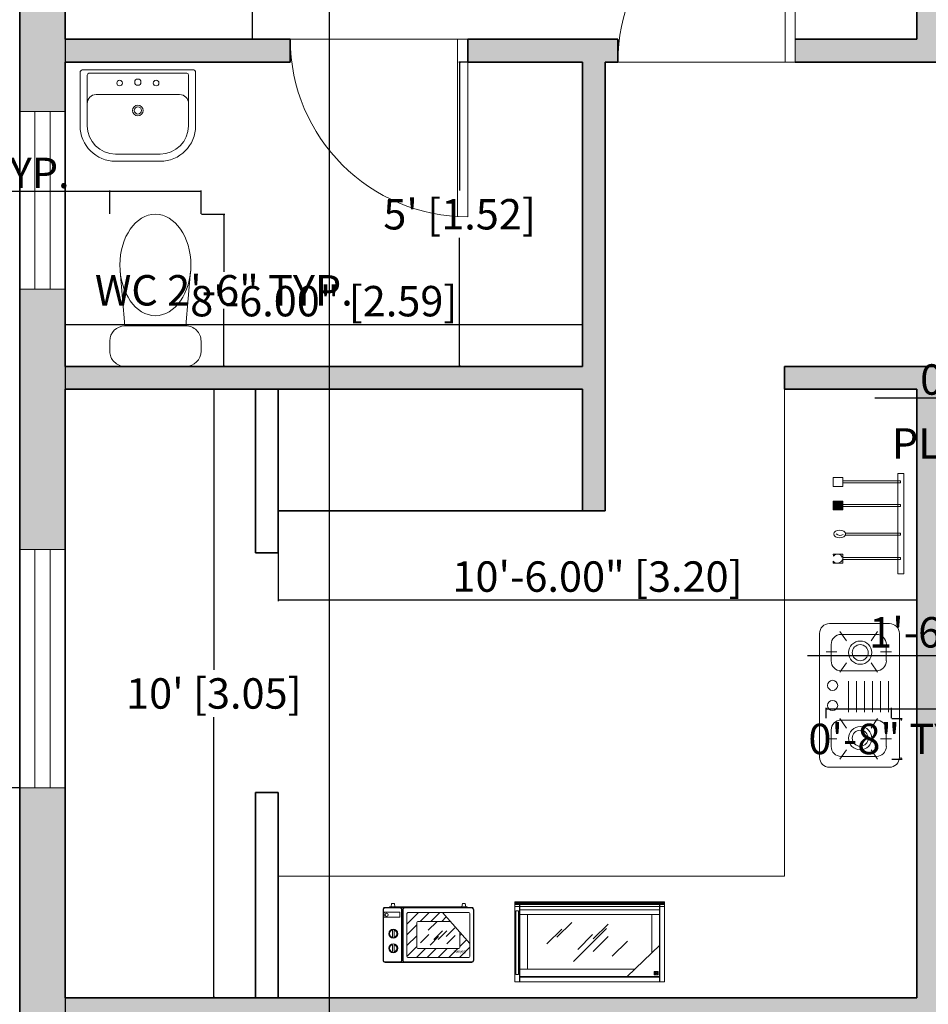
# Model space of a CAD drawing. Units: inches. Extents: x 2322 to 2932, y 142 to 762.
# Tile 4 of 7: x 2430 to 2609, y 376 to 570. Entities that reach past the tile are written whole.
import ezdxf

# ---------------------------------------------------------------- set-up
doc = ezdxf.new("R2010")
doc.units = ezdxf.units.IN
doc.header["$MEASUREMENT"] = 0
for name, color, linetype, lineweight in [('A-ANNO-DIMS', 2, 'Continuous', 18), ('A-ANNO-TEXT', 7, 'Continuous', 15), ('A-DOOR', 3, 'Continuous', 18), ('A-EQPM', 8, 'Continuous', 15), ('A-EQPM-PATT', 8, 'Continuous', 13), ('A-FLOR-CASE', 32, 'Continuous', 18), ('A-FLOR-FIXT', 9, 'Continuous', 18), ('A-GLAZ', 4, 'Continuous', 18), ('A-WALL', 7, 'Continuous', 35)]:
    doc.layers.add(name, color=color, linetype=linetype, lineweight=lineweight)
doc.layers.add('A-WALL-PATT', color=40, linetype='Continuous', lineweight=13, true_color=0xf8d731)
doc.styles.get("Standard").update_dxf_attribs({"font": 'italic8.shx'})
doc.dimstyles.get("Standard").update_dxf_attribs({"dimtxt": 6, "dimasz": 0.15, "dimexe": 0.18, "dimexo": 0.0625, "dimgap": 0.09, "dimtad": 1, "dimtih": 1, "dimtoh": 1, "dimzin": 0, "dimdsep": 46, "dimlunit": 3, "dimtxsty": 'Standard', "dimblk": 'CLOSEDBLANK', "dimcen": 0.09, "dimclrd": 3, "dimclre": 1, "dimclrt": 6, "dimadec": 0, "dimazin": 0, "dimtfac": 1, "dimtofl": 0, "dimtmove": 0, "dimatfit": 3, "dimldrblk": 'DOT', "dimfxl": 1, "dimtolj": 1, "dimtzin": 0, "dimarcsym": 0})

# ---------------------------------------------------------------- blocks, each defined once
blk = doc.blocks.new('_ClosedBlank')
at = {"color": 0, "linetype": 'ByBlock', "lineweight": -2}
for p, q in [((-1, 0.2), (0, 0)), ((-1, 0.2), (-1, -0.2)), ((0, 0), (-1, -0.2))]:
    blk.add_line(p, q, dxfattribs=at)
blk = doc.blocks.new('*D8')
at = {"layer": 'A-ANNO-DIMS', "color": 0, "lineweight": -2, "transparency": 16777216}
for p, q in [((2430, 718.82), (2352.33, 718.82)), ((2352.51, 718.67), (2352.51, 501.45)), ((2352.51, 274.91), (2352.51, 492.13)), ((2430, 274.76), (2352.33, 274.76))]:
    blk.add_line(p, q, dxfattribs=at)
at = {"layer": 'Defpoints', "color": 0, "transparency": 16777216}
for p in [(2430.06, 718.82), (2352.51, 274.76), (2430.06, 274.76)]:
    blk.add_point(p, dxfattribs=at)
at = {"layer": 'A-ANNO-DIMS', "color": 0, "lineweight": -2, "transparency": 16777216, "xscale": 0.15, "yscale": 0.15, "zscale": 0.15}
for p, rotation in [((2352.51, 718.82), 90), ((2352.51, 274.76), 270)]:
    blk.add_blockref('_ClosedBlank', p, dxfattribs=dict(at, rotation=rotation))
at = {"layer": 'A-ANNO-DIMS', "color": 0, "transparency": 16777216, "insert": (2352.51, 496.79), "char_height": 6, "attachment_point": 5}
blk.add_mtext('\\A1;37\'-0.06" [11.28]', dxfattribs=at)
blk = doc.blocks.new('_Dot')
at = {"color": 0, "linetype": 'ByBlock', "lineweight": -2}
blk.add_line((-0.5, 0), (-1, 0), dxfattribs=at)
at = {"color": 0, "linetype": 'ByBlock', "const_width": 0.5}
blk.add_lwpolyline([(-0.25, 0, 1), (0.25, 0, 1)], format="xyb", close=True, dxfattribs=at)
blk = doc.blocks.new('*D9')
at = {"layer": 'A-ANNO-DIMS', "color": 0, "lineweight": -2, "transparency": 16777216}
for p, q in [((2460.73, 709.82), (2476.2, 709.82)), ((2476.02, 709.67), (2476.02, 642.48)), ((2476.02, 565.97), (2476.02, 633.16)), ((2460.73, 565.82), (2476.2, 565.82))]:
    blk.add_line(p, q, dxfattribs=at)
at = {"layer": 'Defpoints', "color": 0, "transparency": 16777216}
for p in [(2460.67, 709.82), (2460.67, 565.82), (2476.02, 565.82)]:
    blk.add_point(p, dxfattribs=at)
at = {"layer": 'A-ANNO-DIMS', "color": 0, "lineweight": -2, "transparency": 16777216, "xscale": 0.15, "yscale": 0.15, "zscale": 0.15}
for p, rotation in [((2476.02, 709.82), 90), ((2476.02, 565.82), 270)]:
    blk.add_blockref('_ClosedBlank', p, dxfattribs=dict(at, rotation=rotation))
at = {"layer": 'A-ANNO-DIMS', "color": 0, "transparency": 16777216, "insert": (2476.02, 637.82), "char_height": 6, "attachment_point": 5}
blk.add_mtext("\\A1;12' [3.66]", dxfattribs=at)
blk = doc.blocks.new('*D14')
at = {"layer": 'A-ANNO-DIMS', "color": 0, "lineweight": -2, "transparency": 16777216}
for p, q in [((2439.06, 531.26), (2439.06, 509.34)), ((2541.06, 531.26), (2541.06, 509.34)), ((2540.91, 509.52), (2439.21, 509.52))]:
    blk.add_line(p, q, dxfattribs=at)
at = {"layer": 'Defpoints', "color": 0, "transparency": 16777216}
for p in [(2439.06, 531.32), (2541.06, 531.32), (2439.06, 509.52)]:
    blk.add_point(p, dxfattribs=at)
at = {"layer": 'A-ANNO-DIMS', "color": 0, "lineweight": -2, "transparency": 16777216, "xscale": 0.15, "yscale": 0.15, "zscale": 0.15, "rotation": 180}
blk.add_blockref('_ClosedBlank', (2439.06, 509.52), dxfattribs=at)
at = {"layer": 'A-ANNO-DIMS', "color": 0, "lineweight": -2, "transparency": 16777216, "xscale": 0.15, "yscale": 0.15, "zscale": 0.15}
blk.add_blockref('_ClosedBlank', (2541.06, 509.52), dxfattribs=at)
at = {"layer": 'A-ANNO-DIMS', "color": 0, "transparency": 16777216, "insert": (2490.06, 514.18), "char_height": 6, "attachment_point": 5}
blk.add_mtext('\\A1;8\'-6.00" [2.59]', dxfattribs=at)
blk = doc.blocks.new('*D15')
at = {"layer": 'A-ANNO-DIMS', "color": 0, "lineweight": -2, "transparency": 16777216}
for p, q in [((2525.45, 561.32), (2516.67, 561.32)), ((2516.85, 561.17), (2516.85, 535.98)), ((2516.85, 501.47), (2516.85, 526.66)), ((2525.45, 501.32), (2516.67, 501.32))]:
    blk.add_line(p, q, dxfattribs=at)
at = {"layer": 'Defpoints', "color": 0, "transparency": 16777216}
for p in [(2525.51, 561.32), (2516.85, 501.32), (2525.51, 501.32)]:
    blk.add_point(p, dxfattribs=at)
at = {"layer": 'A-ANNO-DIMS', "color": 0, "lineweight": -2, "transparency": 16777216, "xscale": 0.15, "yscale": 0.15, "zscale": 0.15}
for p, rotation in [((2516.85, 561.32), 90), ((2516.85, 501.32), 270)]:
    blk.add_blockref('_ClosedBlank', p, dxfattribs=dict(at, rotation=rotation))
at = {"layer": 'A-ANNO-DIMS', "color": 0, "transparency": 16777216, "insert": (2516.85, 531.32), "char_height": 6, "attachment_point": 5}
blk.add_mtext("\\A1;5' [1.52]", dxfattribs=at)
blk = doc.blocks.new('*D16')
at = {"layer": 'A-ANNO-DIMS', "color": 0, "lineweight": -2, "transparency": 16777216}
for p, q in [((2481.06, 469.54), (2481.06, 455.03)), ((2607.06, 469.54), (2607.06, 455.03)), ((2606.91, 455.21), (2481.21, 455.21))]:
    blk.add_line(p, q, dxfattribs=at)
at = {"layer": 'Defpoints', "color": 0, "transparency": 16777216}
for p in [(2481.06, 469.6), (2607.06, 469.6), (2481.06, 455.21)]:
    blk.add_point(p, dxfattribs=at)
at = {"layer": 'A-ANNO-DIMS', "color": 0, "lineweight": -2, "transparency": 16777216, "xscale": 0.15, "yscale": 0.15, "zscale": 0.15, "rotation": 180}
blk.add_blockref('_ClosedBlank', (2481.06, 455.21), dxfattribs=at)
at = {"layer": 'A-ANNO-DIMS', "color": 0, "lineweight": -2, "transparency": 16777216, "xscale": 0.15, "yscale": 0.15, "zscale": 0.15}
blk.add_blockref('_ClosedBlank', (2607.06, 455.21), dxfattribs=at)
at = {"layer": 'A-ANNO-DIMS', "color": 0, "transparency": 16777216, "insert": (2544.06, 459.87), "char_height": 6, "attachment_point": 5}
blk.add_mtext('\\A1;10\'-6.00" [3.20]', dxfattribs=at)
blk = doc.blocks.new('*D17')
at = {"layer": 'A-ANNO-DIMS', "color": 0, "lineweight": -2, "transparency": 16777216}
for p, q in [((2460.37, 496.82), (2468.55, 496.82)), ((2468.37, 496.67), (2468.37, 441.48)), ((2468.37, 376.97), (2468.37, 432.16)), ((2460.37, 376.82), (2468.55, 376.82))]:
    blk.add_line(p, q, dxfattribs=at)
at = {"layer": 'Defpoints', "color": 0, "transparency": 16777216}
for p in [(2460.31, 496.82), (2460.31, 376.82), (2468.37, 376.82)]:
    blk.add_point(p, dxfattribs=at)
at = {"layer": 'A-ANNO-DIMS', "color": 0, "lineweight": -2, "transparency": 16777216, "xscale": 0.15, "yscale": 0.15, "zscale": 0.15}
for p, rotation in [((2468.37, 496.82), 90), ((2468.37, 376.82), 270)]:
    blk.add_blockref('_ClosedBlank', p, dxfattribs=dict(at, rotation=rotation))
at = {"layer": 'A-ANNO-DIMS', "color": 0, "transparency": 16777216, "insert": (2468.37, 436.82), "char_height": 6, "attachment_point": 5}
blk.add_mtext("\\A1;10' [3.05]", dxfattribs=at)
blk = doc.blocks.new('DOOR-SWING-35')
for p, q in [((0, 35), (0, 0)), ((2, 35), (2, 0)), ((0, 0), (35, 0))]:
    blk.add_line(p, q)
blk.add_arc((0, 0), 35, 0, 90)
blk = doc.blocks.new('WINDOW-47X9')
for p, q in [((47, 9), (0, 9)), ((0, 9), (0, 0)), ((47, 0), (47, 9)), ((0, 6), (47, 6)), ((0, 3), (47, 3)), ((0, 0), (47, 0))]:
    blk.add_line(p, q)
blk = doc.blocks.new('WC-TANK')
for p, q in [((3, 18), (5, 18)), ((8, 15), (18.75, 15.95)), ((0, 3), (0, 15)), ((8, 15), (8, 3)), ((8, 3), (18.75, 2.05)), ((5, 0), (3, 0))]:
    blk.add_line(p, q)
for centre, start, end in [((3, 15), 90, 180), ((5, 15), 0, 90), ((3, 3), 180, 270), ((5, 3), 270, 0)]:
    blk.add_arc(centre, 3, start, end)
blk.add_ellipse((20, 9), major_axis=(10, 0), ratio=0.7)
blk = doc.blocks.new('COOKTOP-BURNER')
for p, q in [((2.72, 8.03), (4.01, 6.17)), ((10.17, 8.03), (8.88, 6.17)), ((9.92, 7.46), (2.97, 7.46)), ((0, 4.01), (2.15, 4.01)), ((1, 5.49), (1, 2.25)), ((12.89, 4.01), (10.74, 4.01)), ((11.88, 2.25), (11.88, 5.49)), ((2.72, 0), (4.01, 1.86)), ((2.97, 0.29), (9.92, 0.29)), ((10.17, 0), (8.88, 1.86))]:
    blk.add_line(p, q)
for radius in [2.29, 1.58]:
    blk.add_circle((6.73, 3.87), radius)
for centre, start, end in [((2.97, 5.49), 90, 180), ((9.92, 5.49), 0, 90), ((2.97, 2.25), 180, 270), ((9.92, 2.25), 270, 0)]:
    blk.add_arc(centre, 1.97, start, end)
blk = doc.blocks.new('*D31')
at = {"layer": 'A-ANNO-DIMS', "color": 1, "lineweight": -2, "transparency": 16777216}
for p, q in [((2660.69, 447.24), (2660.69, 444.03)), ((2679.17, 447.24), (2679.17, 444.03))]:
    blk.add_line(p, q, dxfattribs=at)
at = {"layer": 'A-ANNO-DIMS', "color": 3, "lineweight": -2, "transparency": 16777216}
for p, q in [((2660.69, 444.21), (2585.5, 444.21)), ((2679.02, 444.21), (2660.84, 444.21))]:
    blk.add_line(p, q, dxfattribs=at)
at = {"layer": 'Defpoints', "color": 0, "transparency": 16777216}
for p in [(2660.69, 447.3), (2679.17, 447.3), (2660.69, 444.21)]:
    blk.add_point(p, dxfattribs=at)
at = {"layer": 'A-ANNO-DIMS', "color": 3, "lineweight": -2, "transparency": 16777216, "xscale": 0.15, "yscale": 0.15, "zscale": 0.15, "rotation": 180}
blk.add_blockref('_ClosedBlank', (2660.69, 444.21), dxfattribs=at)
at = {"layer": 'A-ANNO-DIMS', "color": 3, "lineweight": -2, "transparency": 16777216, "xscale": 0.15, "yscale": 0.15, "zscale": 0.15}
blk.add_blockref('_ClosedBlank', (2679.17, 444.21), dxfattribs=at)
at = {"layer": 'A-ANNO-DIMS', "color": 6, "transparency": 16777216, "insert": (2623.02, 448.87), "char_height": 6, "attachment_point": 5}
blk.add_mtext('\\A1;1\'-6 1/2" TYP.', dxfattribs=at)
blk = doc.blocks.new('*D32')
at = {"layer": 'A-ANNO-DIMS', "color": 1, "lineweight": -2, "transparency": 16777216}
for p, q in [((2653.34, 493), (2651.16, 493)), ((2653.34, 479.24), (2651.16, 479.24))]:
    blk.add_line(p, q, dxfattribs=at)
at = {"layer": 'A-ANNO-DIMS', "color": 3, "lineweight": -2, "transparency": 16777216}
for p, q in [((2651.34, 492.85), (2651.34, 489.78)), ((2651.34, 479.39), (2651.34, 482.46))]:
    blk.add_line(p, q, dxfattribs=at)
at = {"layer": 'Defpoints', "color": 0, "transparency": 16777216}
for p in [(2653.4, 493), (2651.34, 479.24), (2653.4, 479.24)]:
    blk.add_point(p, dxfattribs=at)
at = {"layer": 'A-ANNO-DIMS', "color": 3, "lineweight": -2, "transparency": 16777216, "xscale": 0.15, "yscale": 0.15, "zscale": 0.15}
for p, rotation in [((2651.34, 493), 90), ((2651.34, 479.24), 270)]:
    blk.add_blockref('_ClosedBlank', p, dxfattribs=dict(at, rotation=rotation))
at = {"layer": 'A-ANNO-DIMS', "color": 6, "transparency": 16777216, "insert": (2651.34, 486.12), "char_height": 6, "attachment_point": 5}
blk.add_mtext('\\A1;PLACE SETTING 1\'-2" TYP.', dxfattribs=at)
blk = doc.blocks.new('*D33')
at = {"layer": 'A-ANNO-DIMS', "color": 1, "lineweight": -2, "transparency": 16777216}
for p, q in [((2653.4, 493.07), (2653.4, 495.25)), ((2662.31, 493.07), (2662.31, 495.25))]:
    blk.add_line(p, q, dxfattribs=at)
at = {"layer": 'A-ANNO-DIMS', "color": 3, "lineweight": -2, "transparency": 16777216}
for p, q in [((2653.4, 495.07), (2598.79, 495.07)), ((2662.16, 495.07), (2653.55, 495.07))]:
    blk.add_line(p, q, dxfattribs=at)
at = {"layer": 'Defpoints', "color": 0, "transparency": 16777216}
for p in [(2653.4, 495.07), (2653.4, 493), (2662.31, 493)]:
    blk.add_point(p, dxfattribs=at)
at = {"layer": 'A-ANNO-DIMS', "color": 3, "lineweight": -2, "transparency": 16777216, "xscale": 0.15, "yscale": 0.15, "zscale": 0.15, "rotation": 180}
blk.add_blockref('_ClosedBlank', (2653.4, 495.07), dxfattribs=at)
at = {"layer": 'A-ANNO-DIMS', "color": 3, "lineweight": -2, "transparency": 16777216, "xscale": 0.15, "yscale": 0.15, "zscale": 0.15}
blk.add_blockref('_ClosedBlank', (2662.31, 495.07), dxfattribs=at)
at = {"layer": 'A-ANNO-DIMS', "color": 6, "transparency": 16777216, "insert": (2626.02, 498.73), "char_height": 6, "attachment_point": 5}
blk.add_mtext('\\A1;0\'-9" TYP.', dxfattribs=at)
blk = doc.blocks.new('*D36')
at = {"layer": 'A-ANNO-DIMS', "color": 1, "lineweight": -2, "transparency": 16777216}
for p, q in [((2465.9, 531.32), (2470.52, 531.32)), ((2465.9, 501.32), (2470.52, 501.32))]:
    blk.add_line(p, q, dxfattribs=at)
at = {"layer": 'A-ANNO-DIMS', "color": 3, "lineweight": -2, "transparency": 16777216}
for p, q in [((2470.34, 531.17), (2470.34, 519.98)), ((2470.34, 501.47), (2470.34, 512.66))]:
    blk.add_line(p, q, dxfattribs=at)
at = {"layer": 'Defpoints', "color": 0, "transparency": 16777216}
for p in [(2465.84, 531.32), (2470.34, 531.32), (2465.84, 501.32)]:
    blk.add_point(p, dxfattribs=at)
at = {"layer": 'A-ANNO-DIMS', "color": 3, "lineweight": -2, "transparency": 16777216, "xscale": 0.15, "yscale": 0.15, "zscale": 0.15}
for p, rotation in [((2470.34, 531.32), 90), ((2470.34, 501.32), 270)]:
    blk.add_blockref('_ClosedBlank', p, dxfattribs=dict(at, rotation=rotation))
at = {"layer": 'A-ANNO-DIMS', "color": 6, "transparency": 16777216, "insert": (2470.34, 516.32), "char_height": 6, "attachment_point": 5}
blk.add_mtext('\\A1;WC 2\'-6" TYP.', dxfattribs=at)
blk = doc.blocks.new('*D37')
at = {"layer": 'A-ANNO-DIMS', "color": 1, "lineweight": -2, "transparency": 16777216}
for p, q in [((2447.84, 531.38), (2447.84, 536)), ((2465.84, 531.38), (2465.84, 536))]:
    blk.add_line(p, q, dxfattribs=at)
at = {"layer": 'A-ANNO-DIMS', "color": 3, "lineweight": -2, "transparency": 16777216}
for p, q in [((2447.84, 535.82), (2395.51, 535.82)), ((2465.69, 535.82), (2447.99, 535.82))]:
    blk.add_line(p, q, dxfattribs=at)
at = {"layer": 'Defpoints', "color": 0, "transparency": 16777216}
for p in [(2447.84, 535.82), (2447.84, 531.32), (2465.84, 531.32)]:
    blk.add_point(p, dxfattribs=at)
at = {"layer": 'A-ANNO-DIMS', "color": 3, "lineweight": -2, "transparency": 16777216, "xscale": 0.15, "yscale": 0.15, "zscale": 0.15, "rotation": 180}
blk.add_blockref('_ClosedBlank', (2447.84, 535.82), dxfattribs=at)
at = {"layer": 'A-ANNO-DIMS', "color": 3, "lineweight": -2, "transparency": 16777216, "xscale": 0.15, "yscale": 0.15, "zscale": 0.15}
blk.add_blockref('_ClosedBlank', (2465.84, 535.82), dxfattribs=at)
at = {"layer": 'A-ANNO-DIMS', "color": 6, "transparency": 16777216, "insert": (2421.6, 539.48), "char_height": 6, "attachment_point": 5}
blk.add_mtext('\\A1;1\'-6" TYP.', dxfattribs=at)
blk = doc.blocks.new('*D42')
at = {"layer": 'A-ANNO-DIMS', "color": 1, "lineweight": -2, "transparency": 16777216}
for p, q in [((2589.15, 431.92), (2589.15, 433.98)), ((2602.04, 431.92), (2602.04, 433.98))]:
    blk.add_line(p, q, dxfattribs=at)
at = {"layer": 'A-ANNO-DIMS', "color": 3, "lineweight": -2, "transparency": 16777216}
for p, q in [((2589.3, 433.8), (2601.89, 433.8)), ((2602.04, 433.8), (2699.51, 433.8))]:
    blk.add_line(p, q, dxfattribs=at)
at = {"layer": 'Defpoints', "color": 0, "transparency": 16777216}
for p in [(2602.04, 433.8), (2589.15, 431.86), (2602.04, 431.86)]:
    blk.add_point(p, dxfattribs=at)
at = {"layer": 'A-ANNO-DIMS', "color": 3, "lineweight": -2, "transparency": 16777216, "xscale": 0.15, "yscale": 0.15, "zscale": 0.15, "rotation": 180}
blk.add_blockref('_ClosedBlank', (2589.15, 433.8), dxfattribs=at)
at = {"layer": 'A-ANNO-DIMS', "color": 3, "lineweight": -2, "transparency": 16777216, "xscale": 0.15, "yscale": 0.15, "zscale": 0.15}
blk.add_blockref('_ClosedBlank', (2602.04, 433.8), dxfattribs=at)
at = {"layer": 'A-ANNO-DIMS', "color": 6, "transparency": 16777216, "insert": (2650.85, 437.46), "char_height": 6, "attachment_point": 5}
blk.add_mtext('\\A1;BURNER 1\'-1" TYP.', dxfattribs=at)
blk = doc.blocks.new('*D43')
at = {"layer": 'A-ANNO-DIMS', "color": 1, "lineweight": -2, "transparency": 16777216}
for p, q in [((2602.1, 431.86), (2604.15, 431.86)), ((2602.1, 423.83), (2604.15, 423.83))]:
    blk.add_line(p, q, dxfattribs=at)
at = {"layer": 'A-ANNO-DIMS', "color": 3, "lineweight": -2, "transparency": 16777216}
for p, q in [((2603.97, 431.71), (2603.97, 431.51)), ((2603.97, 423.98), (2603.97, 424.19))]:
    blk.add_line(p, q, dxfattribs=at)
at = {"layer": 'Defpoints', "color": 0, "transparency": 16777216}
for p in [(2602.04, 431.86), (2602.04, 423.83), (2603.97, 423.83)]:
    blk.add_point(p, dxfattribs=at)
at = {"layer": 'A-ANNO-DIMS', "color": 3, "lineweight": -2, "transparency": 16777216, "xscale": 0.15, "yscale": 0.15, "zscale": 0.15}
for p, rotation in [((2603.97, 431.86), 90), ((2603.97, 423.83), 270)]:
    blk.add_blockref('_ClosedBlank', p, dxfattribs=dict(at, rotation=rotation))
at = {"layer": 'A-ANNO-DIMS', "color": 6, "transparency": 16777216, "insert": (2603.97, 427.85), "char_height": 6, "attachment_point": 5}
blk.add_mtext('\\A1;0\'-8" TYP.', dxfattribs=at)
blk = doc.blocks.new('*D51')
at = {"layer": 'A-ANNO-DIMS', "color": 1, "lineweight": -2, "transparency": 16777216}
for p, q in [((2439.06, 709.76), (2439.06, 146.01)), ((2491.1, 709.76), (2491.1, 146.01))]:
    blk.add_line(p, q, dxfattribs=at)
at = {"layer": 'A-ANNO-DIMS', "color": 3, "lineweight": -2, "transparency": 16777216}
blk.add_line((2439.21, 146.19), (2490.95, 146.19), dxfattribs=at)
at = {"layer": 'Defpoints', "color": 0, "transparency": 16777216}
for p in [(2439.06, 709.82), (2491.1, 709.82), (2491.1, 146.19)]:
    blk.add_point(p, dxfattribs=at)
at = {"layer": 'A-ANNO-DIMS', "color": 3, "lineweight": -2, "transparency": 16777216, "xscale": 0.15, "yscale": 0.15, "zscale": 0.15, "rotation": 180}
blk.add_blockref('_ClosedBlank', (2439.06, 146.19), dxfattribs=at)
at = {"layer": 'A-ANNO-DIMS', "color": 3, "lineweight": -2, "transparency": 16777216, "xscale": 0.15, "yscale": 0.15, "zscale": 0.15}
blk.add_blockref('_ClosedBlank', (2491.1, 146.19), dxfattribs=at)
at = {"layer": 'A-ANNO-DIMS', "color": 6, "transparency": 16777216, "insert": (2465.08, 149.85), "char_height": 6, "attachment_point": 5}
blk.add_mtext('\\A1;4\'-4"', dxfattribs=at)
blk = doc.blocks.new('*D57')
at = {"layer": 'A-ANNO-DIMS', "color": 1, "lineweight": -2, "transparency": 16777216}
for p, q in [((2430, 418.18), (2400.26, 418.18)), ((2439, 367.82), (2400.26, 367.82))]:
    blk.add_line(p, q, dxfattribs=at)
at = {"layer": 'A-ANNO-DIMS', "color": 3, "lineweight": -2, "transparency": 16777216}
for p, q in [((2400.44, 418.03), (2400.44, 397.66)), ((2400.44, 367.97), (2400.44, 388.34))]:
    blk.add_line(p, q, dxfattribs=at)
at = {"layer": 'Defpoints', "color": 0, "transparency": 16777216}
for p in [(2400.44, 418.18), (2430.06, 418.18), (2439.06, 367.82)]:
    blk.add_point(p, dxfattribs=at)
at = {"layer": 'A-ANNO-DIMS', "color": 3, "lineweight": -2, "transparency": 16777216, "xscale": 0.15, "yscale": 0.15, "zscale": 0.15}
for p, rotation in [((2400.44, 418.18), 90), ((2400.44, 367.82), 270)]:
    blk.add_blockref('_ClosedBlank', p, dxfattribs=dict(at, rotation=rotation))
at = {"layer": 'A-ANNO-DIMS', "color": 6, "transparency": 16777216, "insert": (2400.44, 393), "char_height": 6, "attachment_point": 5}
blk.add_mtext('\\A1;4\'-2 1/2"', dxfattribs=at)

msp = doc.modelspace()

# ---------------------------------------------------------------- hatches: boundary and pattern name
at = {"layer": 'A-EQPM-PATT'}
h = msp.add_hatch(dxfattribs=at)
h.set_pattern_fill('ANSI31', color=256, scale=12.00081, style=0)
h.paths.add_polyline_path([(2506.622, 384.77), (2518.669, 384.77), (2518.688, 384.771), (2518.707, 384.773), (2518.726, 384.778), (2518.744, 384.785), (2518.762, 384.793), (2518.778, 384.803), (2518.794, 384.814), (2518.808, 384.827), (2518.821, 384.842), (2518.833, 384.857), (2518.843, 384.874), (2518.851, 384.891), (2518.857, 384.909), (2518.862, 384.928), (2518.865, 384.947), (2518.866, 384.967), (2518.866, 387.478), (2516.897, 389.711), (2516.897, 386.738), (2516.896, 386.719), (2516.894, 386.7), (2516.889, 386.681), (2516.882, 386.663), (2516.874, 386.645), (2516.864, 386.629), (2516.853, 386.613), (2516.84, 386.599), (2516.825, 386.586), (2516.81, 386.574), (2516.793, 386.565), (2516.776, 386.556), (2516.758, 386.55), (2516.739, 386.545), (2516.72, 386.542), (2516.701, 386.541), (2508.59, 386.541), (2508.571, 386.542), (2508.552, 386.545), (2508.533, 386.55), (2508.515, 386.556), (2508.498, 386.565), (2508.481, 386.574), (2508.465, 386.586), (2508.451, 386.599), (2508.438, 386.613), (2508.427, 386.629), (2508.417, 386.645), (2508.408, 386.663), (2508.402, 386.681), (2508.397, 386.7), (2508.394, 386.719), (2508.393, 386.738), (2508.393, 391.659), (2508.394, 391.679), (2508.397, 391.698), (2508.402, 391.717), (2508.408, 391.735), (2508.417, 391.752), (2508.427, 391.769), (2508.438, 391.784), (2508.451, 391.799), (2508.465, 391.812), (2508.481, 391.823), (2508.498, 391.833), (2508.515, 391.841), (2508.533, 391.848), (2508.552, 391.852), (2508.571, 391.855), (2508.59, 391.856), (2515.006, 391.856), (2513.444, 393.628), (2506.622, 393.628), (2506.603, 393.627), (2506.583, 393.624), (2506.565, 393.619), (2506.547, 393.613), (2506.529, 393.605), (2506.512, 393.595), (2506.497, 393.583), (2506.483, 393.57), (2506.47, 393.556), (2506.458, 393.54), (2506.448, 393.524), (2506.44, 393.506), (2506.433, 393.488), (2506.429, 393.469), (2506.426, 393.45), (2506.425, 393.431), (2506.425, 384.967), (2506.426, 384.947), (2506.429, 384.928), (2506.433, 384.909), (2506.44, 384.891), (2506.448, 384.874), (2506.458, 384.857), (2506.47, 384.842), (2506.483, 384.827), (2506.497, 384.814), (2506.512, 384.803), (2506.529, 384.793), (2506.547, 384.785), (2506.565, 384.778), (2506.583, 384.773), (2506.603, 384.771)])
at = {"layer": 'A-WALL-PATT'}
h = msp.add_hatch(color=256, dxfattribs=at)
h.dxf.hatch_style = 1
h.paths.add_polyline_path([(2439.065, 709.819), (2491.097, 709.819), (2491.097, 718.819), (2430.065, 718.819), (2430.065, 663.548), (2439.065, 663.548)])
h.paths.add_polyline_path([(2704.233, 718.819), (2654.246, 718.819), (2654.246, 709.819), (2668.565, 709.819), (2668.565, 661.819), (2673.065, 661.819), (2673.065, 709.819), (2704.233, 709.819)], flags=17)
h.paths.add_polyline_path([(2624.246, 718.819), (2538.097, 718.819), (2538.097, 709.819), (2607.065, 709.819), (2607.065, 565.819), (2583.065, 565.819), (2583.065, 561.319), (2611.565, 561.319), (2611.565, 609.319), (2668.565, 609.319), (2668.565, 561.319), (2758.065, 561.319), (2758.065, 565.819), (2673.065, 565.819), (2673.065, 626.819), (2668.565, 626.819), (2668.565, 613.819), (2611.565, 613.819), (2611.565, 709.819), (2624.246, 709.819)])
h.paths.add_polyline_path([(2802.065, 718.819), (2751.233, 718.819), (2751.233, 709.819), (2793.065, 709.819), (2793.065, 660.138), (2802.065, 660.138)])
h.paths.add_polyline_path([(2802.065, 613.138), (2793.065, 613.138), (2793.065, 478.568), (2802.065, 478.568)])
h.paths.add_polyline_path([(2439.065, 616.548), (2430.065, 616.548), (2430.065, 551.562), (2439.065, 551.562), (2439.065, 561.319), (2483.455, 561.319), (2483.455, 565.819), (2439.065, 565.819)])
h.paths.add_polyline_path([(2548.065, 565.819), (2518.455, 565.819), (2518.455, 561.319), (2541.065, 561.319), (2541.065, 501.319), (2439.065, 501.319), (2439.065, 516.562), (2430.065, 516.562), (2430.065, 465.181), (2439.065, 465.181), (2439.065, 496.819), (2503.266, 496.819), (2541.065, 496.819), (2541.065, 472.819), (2545.565, 472.819), (2545.565, 561.319), (2548.065, 561.319)])
h.paths.add_polyline_path([(2439.065, 418.181), (2430.065, 418.181), (2430.065, 342.453), (2439.065, 342.453), (2439.065, 367.819), (2602.565, 367.819), (2602.565, 283.756), (2594.693, 283.756), (2594.693, 274.756), (2611.565, 274.756), (2611.565, 501.319), (2580.942, 501.319), (2580.942, 496.819), (2607.065, 496.819), (2607.065, 376.819), (2439.065, 376.819)])
h.paths.add_polyline_path([(2793.057, 530.805), (2793.057, 530.68), (2793.106, 530.68), (2793.106, 530.805)], flags=25)
h.paths.add_polyline_path([(2793.057, 530.808), (2793.057, 530.676), (2793.106, 530.676), (2793.106, 530.808)], flags=9)

# ---------------------------------------------------------------- linework, layer by layer
at = {"layer": 'A-EQPM'}
for p, q in [((2603.325, 480.18), (2604.462, 480.18)), ((2603.325, 460.41), (2603.325, 480.18)), ((2604.462, 480.18), (2604.462, 460.41)), ((2590.568, 477.65), (2590.568, 479.382)), ((2590.568, 479.382), (2592.466, 479.382)), ((2592.466, 479.382), (2592.466, 477.65)), ((2592.468, 478.34), (2592.468, 478.754)), ((2592.468, 478.754), (2603.841, 478.754)), ((2603.841, 478.34), (2592.468, 478.34)), ((2603.841, 478.754), (2603.841, 478.34)), ((2592.466, 477.65), (2590.568, 477.65)), ((2590.568, 474.735), (2592.466, 474.735)), ((2590.568, 474.735), (2590.568, 473.003)), ((2590.568, 474.449), (2590.568, 474.522)), ((2590.568, 474.522), (2592.466, 474.522)), ((2592.466, 474.449), (2590.568, 474.449)), ((2590.568, 474.243), (2590.568, 474.315)), ((2590.568, 474.315), (2592.456, 474.315)), ((2592.456, 474.243), (2590.568, 474.243)), ((2590.568, 474.025), (2590.568, 474.098)), ((2590.568, 474.098), (2592.466, 474.098)), ((2592.466, 474.025), (2590.568, 474.025)), ((2590.568, 473.819), (2590.568, 473.891)), ((2590.568, 473.891), (2592.456, 473.891)), ((2592.456, 473.819), (2590.568, 473.819)), ((2592.456, 474.315), (2592.456, 474.243)), ((2592.456, 473.891), (2592.456, 473.819)), ((2592.466, 474.735), (2592.466, 473.003)), ((2592.466, 474.522), (2592.466, 474.449)), ((2592.466, 474.098), (2592.466, 474.025)), ((2592.468, 473.693), (2592.468, 474.107)), ((2592.468, 474.107), (2603.841, 474.107)), ((2603.841, 474.107), (2603.841, 473.693)), ((2590.568, 473.581), (2590.568, 473.653)), ((2590.568, 473.653), (2592.456, 473.653)), ((2592.456, 473.581), (2590.568, 473.581)), ((2590.579, 473.364), (2590.568, 473.436)), ((2590.568, 473.436), (2592.466, 473.436)), ((2590.568, 473.003), (2590.568, 473.383)), ((2590.568, 473.157), (2590.568, 473.229)), ((2590.568, 473.229), (2592.456, 473.229)), ((2592.456, 473.157), (2590.568, 473.157)), ((2592.466, 473.003), (2590.568, 473.003)), ((2592.466, 473.364), (2590.579, 473.364)), ((2592.456, 473.653), (2592.456, 473.581)), ((2592.456, 473.229), (2592.456, 473.157)), ((2592.466, 473.436), (2592.466, 473.364)), ((2603.841, 473.693), (2592.468, 473.693)), ((2603.841, 468.045), (2592.944, 468.045)), ((2592.956, 468.46), (2603.841, 468.46)), ((2603.841, 468.46), (2603.841, 468.045)), ((2590.609, 463.921), (2590.568, 464.259)), ((2590.568, 464.259), (2592.466, 464.259)), ((2592.466, 464.259), (2592.466, 462.527)), ((2590.568, 462.527), (2590.568, 462.907)), ((2592.466, 462.527), (2590.568, 462.527)), ((2592.468, 463.217), (2592.468, 463.631)), ((2592.468, 463.631), (2603.841, 463.631)), ((2603.841, 463.217), (2592.468, 463.217)), ((2603.841, 463.631), (2603.841, 463.217)), ((2604.462, 460.41), (2603.325, 460.41)), ((2589.829, 450.602), (2601.64, 450.602)), ((2587.861, 424.224), (2587.861, 448.633)), ((2603.609, 448.633), (2603.609, 424.224)), ((2593.589, 439.274), (2593.589, 433.108)), ((2595.164, 439.274), (2595.164, 433.108)), ((2596.739, 439.274), (2596.739, 433.108)), ((2598.314, 439.274), (2598.314, 433.108)), ((2599.888, 439.274), (2599.888, 433.108)), ((2601.463, 439.274), (2601.463, 433.108)), ((2601.64, 422.255), (2589.829, 422.255)), ((2501.74, 394.218), (2501.74, 384.179)), ((2501.819, 394.218), (2501.819, 384.179)), ((2505.086, 394.612), (2502.134, 394.612)), ((2505.086, 394.533), (2502.134, 394.533)), ((2502.921, 394.612), (2503.118, 394.77)), ((2504.299, 394.77), (2503.118, 394.77)), ((2503.338, 394.77), (2503.433, 395.4)), ((2503.984, 395.4), (2503.433, 395.4)), ((2504.079, 394.77), (2503.984, 395.4)), ((2517.094, 394.77), (2504.299, 394.77)), ((2506.031, 394.612), (2505.086, 394.612)), ((2505.401, 394.218), (2505.401, 384.179)), ((2505.48, 394.218), (2505.48, 384.179)), ((2505.638, 394.218), (2505.638, 384.179)), ((2505.716, 394.218), (2505.716, 384.179)), ((2519.26, 394.612), (2506.031, 394.612)), ((2519.26, 394.533), (2506.031, 394.533)), ((2518.275, 394.77), (2517.094, 394.77)), ((2517.315, 394.77), (2517.409, 395.4)), ((2517.96, 395.4), (2517.409, 395.4)), ((2518.055, 394.77), (2517.96, 395.4)), ((2518.275, 394.77), (2518.472, 394.612)), ((2519.575, 384.179), (2519.575, 394.218)), ((2519.653, 384.179), (2519.653, 394.218)), ((2557.278, 395.707), (2527.751, 395.707)), ((2527.751, 395.707), (2527.751, 379.959)), ((2528.656, 395.653), (2527.751, 395.653)), ((2528.656, 395.559), (2527.751, 395.559)), ((2528.656, 395.423), (2527.751, 395.423)), ((2528.656, 395.18), (2527.751, 395.18)), ((2528.656, 394.815), (2527.751, 394.815)), ((2528.656, 395.707), (2528.656, 379.959)), ((2528.735, 395.707), (2528.735, 379.959)), ((2556.294, 395.653), (2528.735, 395.653)), ((2556.294, 395.559), (2528.735, 395.559)), ((2556.294, 395.423), (2528.735, 395.423)), ((2556.294, 395.18), (2528.735, 395.18)), ((2556.294, 394.815), (2528.735, 394.815)), ((2556.294, 379.959), (2556.294, 395.707)), ((2556.373, 379.959), (2556.373, 395.707)), ((2557.278, 395.653), (2556.373, 395.653)), ((2557.278, 395.559), (2556.373, 395.559)), ((2557.278, 395.423), (2556.373, 395.423)), ((2557.278, 395.18), (2556.373, 395.18)), ((2557.278, 394.815), (2556.373, 394.815)), ((2557.278, 379.959), (2557.278, 395.707)), ((2501.898, 393.508), (2501.898, 392.682)), ((2501.898, 392.682), (2505.048, 392.682)), ((2505.048, 393.666), (2502.056, 393.666)), ((2505.048, 392.682), (2505.048, 393.666)), ((2506.425, 393.431), (2506.425, 384.967)), ((2518.669, 393.628), (2506.622, 393.628)), ((2518.866, 387.478), (2513.444, 393.628)), ((2518.866, 384.967), (2518.866, 393.431)), ((2527.945, 381.401), (2527.945, 393.94)), ((2527.945, 393.94), (2528.467, 393.94)), ((2528.467, 393.94), (2528.467, 381.401)), ((2556.294, 394.132), (2528.735, 394.132)), ((2556.294, 393.226), (2528.735, 393.226)), ((2530.231, 393.226), (2530.231, 382.439)), ((2554.798, 385.699), (2554.798, 393.226)), ((2508.393, 391.659), (2508.393, 386.738)), ((2515.006, 391.856), (2508.59, 391.856)), ((2512.35, 391.808), (2510.659, 390.117)), ((2515.92, 390.602), (2514.229, 388.911)), ((2537.02, 390.362), (2534.086, 387.428)), ((2538.987, 391.672), (2536.053, 388.739)), ((2545.86, 390.47), (2539.336, 383.946)), ((2546.144, 391.345), (2543.211, 388.411)), ((2503.598, 388.84), (2503.598, 390.05)), ((2503.913, 388.84), (2503.913, 390.05)), ((2510.795, 389.31), (2509.105, 387.619)), ((2512.716, 388.884), (2511.025, 387.193)), ((2513.478, 390.011), (2511.787, 388.32)), ((2514.319, 389.977), (2512.629, 388.286)), ((2515.993, 389.112), (2514.302, 387.421)), ((2516.897, 386.738), (2516.897, 389.711)), ((2543.085, 389.27), (2540.151, 386.336)), ((2546.144, 388.888), (2543.211, 385.954)), ((2503.598, 385.97), (2503.598, 387.18)), ((2503.913, 385.97), (2503.913, 387.18)), ((2508.59, 386.541), (2516.701, 386.541)), ((2549.968, 387.998), (2546.957, 384.987)), ((2556.373, 387.21), (2549.923, 381.022)), ((2506.622, 384.77), (2518.669, 384.77)), ((2505.086, 383.864), (2502.134, 383.864)), ((2505.086, 383.785), (2502.134, 383.785)), ((2506.031, 383.785), (2504.56, 383.785)), ((2506.031, 383.864), (2519.26, 383.864)), ((2506.031, 383.785), (2519.26, 383.785)), ((2528.467, 381.401), (2527.945, 381.401)), ((2528.735, 382.439), (2551.4, 382.439)), ((2528.735, 381.022), (2556.294, 381.022)), ((2528.735, 380.864), (2556.294, 380.864)), ((2556.004, 381.321), (2555.258, 381.968)), ((2556.004, 381.968), (2555.258, 381.321)), ((2555.258, 381.321), (2555.258, 381.968)), ((2555.258, 381.968), (2556.004, 381.968)), ((2555.258, 381.589), (2555.505, 381.589)), ((2555.258, 381.511), (2555.476, 381.511)), ((2555.258, 381.432), (2555.386, 381.432)), ((2555.258, 381.353), (2555.295, 381.353)), ((2556.004, 381.321), (2555.258, 381.321)), ((2555.269, 381.958), (2555.269, 381.589)), ((2555.348, 381.89), (2555.348, 381.589)), ((2555.427, 381.821), (2555.427, 381.589)), ((2555.505, 381.753), (2555.505, 381.589)), ((2555.505, 381.747), (2555.513, 381.747)), ((2555.505, 381.668), (2555.603, 381.668)), ((2555.505, 381.589), (2555.567, 381.589)), ((2555.505, 381.589), (2555.505, 381.536)), ((2555.658, 381.668), (2555.978, 381.668)), ((2555.694, 381.589), (2555.978, 381.589)), ((2555.742, 381.589), (2555.742, 381.548)), ((2555.749, 381.747), (2555.978, 381.747)), ((2555.82, 381.589), (2555.82, 381.48)), ((2555.84, 381.826), (2555.978, 381.826)), ((2555.899, 381.589), (2555.899, 381.412)), ((2555.93, 381.904), (2555.978, 381.904)), ((2555.978, 381.945), (2555.978, 381.589)), ((2555.978, 381.589), (2556.004, 381.589)), ((2555.978, 381.589), (2555.978, 381.343)), ((2555.978, 381.511), (2556.004, 381.511)), ((2555.978, 381.432), (2556.004, 381.432)), ((2555.978, 381.353), (2556.004, 381.353)), ((2556.004, 381.968), (2556.004, 381.321)), ((2527.751, 379.959), (2557.278, 379.959))]:
    msp.add_line(p, q, dxfattribs=at)
for centre, radius in [((2590.438, 438.413), 1.004), ((2590.438, 434.443), 1.004), ((2502.446, 393.165), 0.314), ((2503.756, 389.445), 0.886), ((2503.756, 389.445), 0.846), ((2503.756, 386.575), 0.886), ((2503.756, 386.575), 0.846)]:
    msp.add_circle(centre, radius, dxfattribs=at)
for centre, radius, start, end in [((2591.916, 469.149), 1.164, 229.28003, 300.31399), ((2591.396, 463.21), 1.06, 25.53866, 137.91532), ((2591.387, 463.597), 1.07, 220.12991, 338.3923), ((2589.829, 448.633), 1.968, 90, 180), ((2601.64, 448.633), 1.968, 0, 90), ((2589.829, 424.224), 1.968, 180, 270), ((2601.64, 424.224), 1.968, 270, 0), ((2502.134, 394.218), 0.394, 90, 180), ((2502.134, 394.218), 0.315, 90, 180), ((2505.086, 394.218), 0.394, 0, 90), ((2505.086, 394.218), 0.315, 0, 90), ((2506.031, 394.218), 0.394, 90, 180), ((2506.031, 394.218), 0.315, 90, 180), ((2519.26, 394.218), 0.394, 0, 90), ((2519.26, 394.218), 0.315, 0, 90), ((2502.056, 393.508), 0.157, 90, 180), ((2506.622, 393.431), 0.197, 90, 180), ((2518.669, 393.431), 0.197, 0, 90), ((2508.59, 391.659), 0.197, 90, 180), ((2503.756, 389.445), 0.728, 111.32369, 248.67631), ((2503.519, 390.05), 0.0787, 0, 111.32369), ((2503.519, 388.84), 0.0787, 248.67631, 0), ((2503.992, 390.05), 0.0787, 68.67631, 180), ((2503.992, 388.84), 0.0787, 180, 291.32369), ((2503.756, 389.445), 0.728, 291.32369, 68.67631), ((2503.756, 386.575), 0.728, 111.32369, 248.67631), ((2503.519, 387.18), 0.0787, 0, 111.32369), ((2503.992, 387.18), 0.0787, 68.67631, 180), ((2503.756, 386.575), 0.728, 291.32369, 68.67631), ((2508.59, 386.738), 0.197, 180, 270), ((2516.701, 386.738), 0.197, 270, 0), ((2503.519, 385.97), 0.0787, 248.67631, 0), ((2503.992, 385.97), 0.0787, 180, 291.32369), ((2506.622, 384.967), 0.197, 180, 270), ((2518.669, 384.967), 0.197, 270, 0), ((2502.134, 384.179), 0.394, 180, 270), ((2502.134, 384.179), 0.315, 180, 270), ((2505.086, 384.179), 0.394, 270, 0), ((2505.086, 384.179), 0.315, 270, 0), ((2506.031, 384.179), 0.394, 180, 270), ((2506.031, 384.179), 0.315, 180, 270), ((2519.26, 384.179), 0.394, 270, 0), ((2519.26, 384.179), 0.315, 270, 0)]:
    msp.add_arc(centre, radius, start, end, dxfattribs=at)
msp.add_ellipse((2591.83, 468.266), major_axis=(1.163, 0), ratio=0.6589774, dxfattribs=at)
at = {"layer": 'A-FLOR-CASE'}
for p, q in [((2583.065, 561.319), (2583.065, 709.819)), ((2580.942, 400.819), (2580.942, 496.819)), ((2481.065, 400.819), (2580.942, 400.819))]:
    msp.add_line(p, q, dxfattribs=at)
at = {"layer": 'A-FLOR-FIXT'}
for p, q in [((2442.607, 559.829), (2464.145, 559.829)), ((2441.975, 559.197), (2441.975, 548.779)), ((2443.378, 558.776), (2443.378, 553.164)), ((2443.729, 559.127), (2463.022, 559.127)), ((2463.373, 558.776), (2463.373, 553.164)), ((2464.776, 559.197), (2464.776, 548.779)), ((2445.132, 554.918), (2461.619, 554.918)), ((2443.378, 553.164), (2443.378, 548.779)), ((2463.373, 553.164), (2463.373, 548.779)), ((2448.991, 543.166), (2457.761, 543.166)), ((2448.991, 541.763), (2457.761, 541.763))]:
    msp.add_line(p, q, dxfattribs=at)
for centre, radius in [((2449.78, 557.198), 0.561), ((2453.376, 557.373), 0.614), ((2456.971, 557.198), 0.561), ((2453.376, 551.784), 1.052), ((2453.376, 551.784), 0.702)]:
    msp.add_circle(centre, radius, dxfattribs=at)
for centre, radius, start, end in [((2442.607, 559.197), 0.631, 90, 180), ((2464.145, 559.197), 0.631, 0, 90), ((2443.729, 558.776), 0.351, 90, 180), ((2463.022, 558.776), 0.351, 0, 90), ((2445.132, 553.164), 1.754, 90, 180), ((2461.619, 553.164), 1.754, 0, 90), ((2448.991, 548.779), 7.016, 180, 270), ((2448.991, 548.779), 5.613, 180, 270), ((2457.761, 548.779), 7.016, 270, 0), ((2457.761, 548.779), 5.613, 270, 0)]:
    msp.add_arc(centre, radius, start, end, dxfattribs=at)
at = {"layer": 'A-GLAZ'}
for p, q in [((2439.065, 551.562), (2430.065, 551.562)), ((2430.065, 551.562), (2430.065, 516.562)), ((2433.065, 551.562), (2433.065, 516.562)), ((2436.065, 551.562), (2436.065, 516.562)), ((2439.065, 516.562), (2439.065, 551.562)), ((2430.065, 516.562), (2439.065, 516.562))]:
    msp.add_line(p, q, dxfattribs=at)
at = {"layer": 'A-WALL'}
for p, q in [((2430.065, 718.819), (2430.065, 274.756)), ((2439.065, 709.819), (2439.065, 565.819)), ((2607.065, 709.819), (2607.065, 565.819)), ((2483.455, 565.819), (2439.065, 565.819)), ((2483.455, 565.819), (2483.455, 561.319)), ((2548.065, 565.819), (2518.455, 565.819)), ((2518.455, 565.819), (2518.455, 561.319)), ((2548.065, 561.319), (2548.065, 565.819)), ((2607.065, 565.819), (2583.065, 565.819)), ((2607.065, 565.819), (2583.065, 565.819)), ((2439.065, 561.319), (2439.065, 501.319)), ((2483.455, 561.319), (2439.065, 561.319)), ((2541.065, 561.319), (2518.455, 561.319)), ((2541.065, 561.319), (2541.065, 501.319)), ((2545.565, 561.319), (2545.565, 472.819)), ((2548.065, 561.319), (2545.565, 561.319)), ((2611.565, 561.319), (2583.065, 561.319)), ((2541.065, 501.319), (2439.065, 501.319)), ((2611.565, 501.319), (2580.942, 501.319)), ((2580.942, 496.819), (2580.942, 501.319)), ((2439.065, 496.819), (2439.065, 376.819)), ((2503.266, 496.819), (2439.065, 496.819)), ((2476.565, 496.819), (2476.565, 464.561)), ((2481.065, 496.819), (2481.065, 464.561)), ((2541.065, 496.819), (2503.266, 496.819)), ((2541.065, 496.819), (2541.065, 472.819)), ((2607.065, 496.819), (2580.942, 496.819)), ((2607.065, 496.819), (2607.065, 376.819)), ((2545.565, 472.819), (2481.065, 472.819)), ((2481.065, 464.561), (2476.565, 464.561)), ((2481.065, 417.26), (2476.565, 417.26)), ((2476.565, 417.26), (2476.565, 376.819)), ((2481.065, 417.26), (2481.065, 376.819)), ((2607.065, 376.819), (2439.065, 376.819))]:
    msp.add_line(p, q, dxfattribs=at)

# ---------------------------------------------------------------- block references
at = {"layer": 'A-DOOR', "extrusion": (0, 0, -1), "zscale": -1}
msp.add_blockref('DOOR-SWING-35', (-2583.064, 561.319), dxfattribs=at)
at = {"layer": 'A-DOOR', "rotation": 180}
msp.add_blockref('DOOR-SWING-35', (2518.455, 565.818), dxfattribs=at)
at = {"layer": 'A-EQPM'}
msp.add_blockref('COOKTOP-BURNER', (2589.149, 440.995), dxfattribs=at)
at = {"layer": 'A-EQPM', "extrusion": (0, 0, -1), "zscale": -1, "rotation": 180}
msp.add_blockref('COOKTOP-BURNER', (-2589.149, 431.862), dxfattribs=at)
at = {"layer": 'A-FLOR-FIXT', "rotation": 90.0000000000001}
msp.add_blockref('WC-TANK', (2465.836, 501.319), dxfattribs=at)
at = {"layer": 'A-GLAZ', "rotation": 90.00000000000188}
msp.add_blockref('WINDOW-47X9', (2439.064, 418.181), dxfattribs=at)

# ---------------------------------------------------------------- texts
at = {"layer": 'A-ANNO-TEXT'}
msp.add_text('Galanz', height=0.5644, rotation=180, dxfattribs=at).set_placement((2518.124, 386.106))

# ---------------------------------------------------------------- dimensions: what is measured, and where the dimension line sits
at = {"layer": 'A-ANNO-DIMS'}
for base, p1, p2, override, picture, middle in [((2352.512, 274.756), (2430.065, 718.819), (2430.065, 274.756), {"dimclrd": 0, "dimclre": 0, "dimclrt": 0}, '*D8', (2352.512, 496.787)), ((2476.019, 565.819), (2460.669, 709.819), (2460.669, 565.819), {"dimclrd": 0, "dimclre": 0, "dimclrt": 0}, '*D9', (2476.019, 637.819)), ((2516.849, 501.319), (2525.511, 561.319), (2525.511, 501.319), {"dimclrd": 0, "dimclre": 0, "dimclrt": 0}, '*D15', (2516.849, 531.319)), ((2468.372, 376.819), (2460.312, 496.819), (2460.312, 376.819), {"dimclrd": 0, "dimclre": 0, "dimclrt": 0}, '*D17', (2468.372, 436.819)), ((2400.44, 418.181), (2439.065, 367.819), (2430.065, 418.181), {"dimdec": 1, "dimlfac": 1, "dimrnd": 0, "dimzin": 1, "dimdsep": 46, "dimlunit": 4, "dimfrac": 2}, '*D57', (2400.44, 393))]:
    dim = msp.add_linear_dim(base=base, p1=p1, p2=p2, angle=90, dimstyle='Standard', override=override, dxfattribs=at)
    dim.commit()
    dim.dimension.update_dxf_attribs({"geometry": picture, "text_midpoint": middle})
for base, p1, p2, override, picture, middle in [((2491.097, 146.194), (2439.065, 709.819), (2491.097, 709.819), {"dimdec": 1, "dimlfac": 1, "dimrnd": 0, "dimzin": 1, "dimdsep": 46, "dimlunit": 4, "dimfrac": 2}, '*D51', (2465.081, 149.855)), ((2439.065, 509.516), (2541.065, 531.319), (2439.065, 531.319), {"dimclrd": 0, "dimclre": 0, "dimclrt": 0}, '*D14', (2490.065, 514.177)), ((2481.065, 455.205), (2607.065, 469.603), (2481.065, 469.603), {"dimclrd": 0, "dimclre": 0, "dimclrt": 0}, '*D16', (2544.065, 459.867))]:
    dim = msp.add_linear_dim(base=base, p1=p1, p2=p2, dimstyle='Standard', override=override, dxfattribs=at)
    dim.commit()
    dim.dimension.update_dxf_attribs({"geometry": picture, "text_midpoint": middle})
for base, p1, p2, angle, text, picture, middle in [((2447.837, 535.819), (2465.837, 531.319), (2447.837, 531.319), 180, '<> TYP.', '*D37', (2421.597, 539.48)), ((2470.337, 531.319), (2465.837, 501.319), (2465.837, 531.319), 90, 'WC <> TYP.', '*D36', (2470.337, 516.319)), ((2653.405, 495.067), (2662.308, 493.003), (2653.405, 493.003), 180, '<> TYP.', '*D33', (2626.022, 498.729)), ((2651.341, 479.242), (2653.405, 493.003), (2653.405, 479.242), 270, 'PLACE SETTING <> TYP.', '*D32', (2651.341, 486.122)), ((2660.687, 444.207), (2679.166, 447.298), (2660.687, 447.298), 180, '<> TYP.', '*D31', (2623.019, 448.868)), ((2603.969, 423.833), (2602.036, 431.862), (2602.036, 423.833), 270, '<> TYP.', '*D43', (2603.969, 427.848))]:
    dim = msp.add_linear_dim(base=base, p1=p1, p2=p2, angle=angle, text=text, dimstyle='Standard', override={"dimdec": 1, "dimlfac": 1, "dimrnd": 0, "dimzin": 1, "dimdsep": 46, "dimlunit": 4, "dimfrac": 2}, dxfattribs=at)
    dim.commit()
    dim.dimension.update_dxf_attribs({"geometry": picture, "text_midpoint": middle})
dim = msp.add_linear_dim(base=(2602.036, 433.795), p1=(2589.149, 431.862), p2=(2602.036, 431.862), text='BURNER <> TYP.', dimstyle='Standard', override={"dimdec": 1, "dimlfac": 1, "dimrnd": 0, "dimzin": 1, "dimdsep": 46, "dimlunit": 4, "dimfrac": 2}, dxfattribs=at)
dim.commit()
dim.dimension.update_dxf_attribs({"geometry": '*D42', "text_midpoint": (2650.847, 437.457)})

doc.saveas('drawing.dxf')
